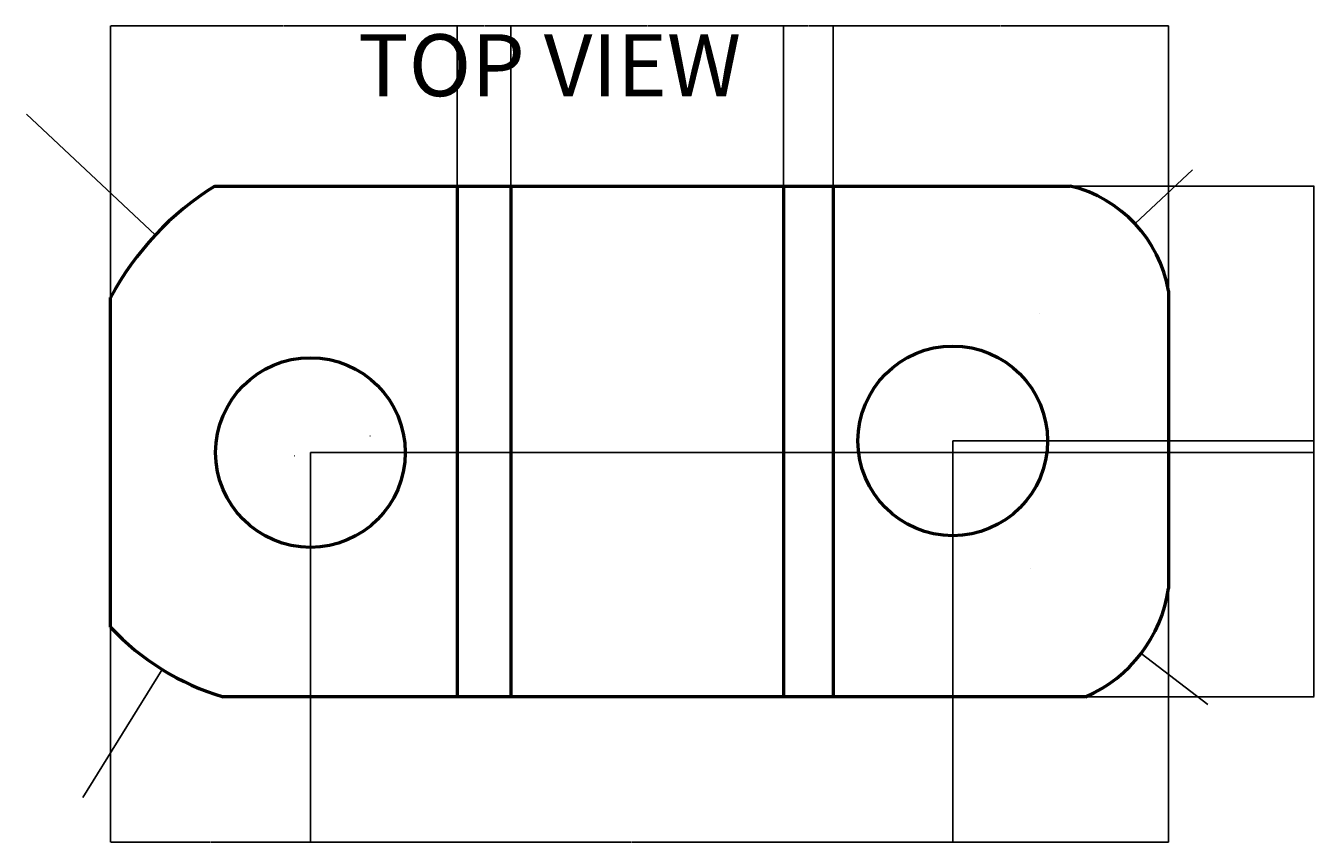
# Model space of a CAD drawing. Units: millimetres. Extents: x 647 to 5260, y 1116 to 2302.
# Tile 2 of 2: x 3387 to 5260, y 1116 to 2302. Entities that reach past the tile are written whole.
import ezdxf

# ---------------------------------------------------------------- set-up
doc = ezdxf.new("R2010")
doc.units = ezdxf.units.MM
for name, color, linetype, lineweight in [('M-DIMS', 2, 'Continuous', 18), ('M-OUTL', 7, 'Continuous', 50), ('M-TEXT', 3, 'Continuous', 25)]:
    doc.layers.add(name, color=color, linetype=linetype, lineweight=lineweight)
doc.styles.get("Standard").update_dxf_attribs({"font": 'arial.ttf'})
doc.dimstyles.get("Standard").update_dxf_attribs({"dimtxt": 0.18, "dimasz": 0.18, "dimexe": 0.18, "dimexo": 0.0625, "dimgap": 0.09, "dimtad": 0, "dimtih": 1, "dimtoh": 1, "dimdec": 4, "dimzin": 0, "dimdsep": 46, "dimtxsty": 'Standard', "dimcen": 0.09, "dimadec": 0, "dimazin": 0, "dimtfac": 1, "dimtdec": 4, "dimtofl": 0, "dimtmove": 0, "dimatfit": 3, "dimfxl": 1, "dimtolj": 1, "dimtzin": 0, "dimarcsym": 0})

# ---------------------------------------------------------------- blocks, each defined once
blk = doc.blocks.new('*D22')
at = {"layer": 'Defpoints', "color": 0, "transparency": 16777216}
for p in [(3800.8, 1681.9), (3510.3, 1428.3), (3800.8, 1116)]:
    blk.add_point(p, dxfattribs=at)
at = {"layer": 'M-DIMS', "color": 0, "lineweight": -2, "transparency": 16777216}
for p, q in [((3800.8, 1681.9), (3800.8, 1115.8)), ((3510.3, 1428.3), (3510.3, 1115.8)), ((3510.5, 1116), (3655.1, 1116)), ((3800.6, 1116), (3656, 1116))]:
    blk.add_line(p, q, dxfattribs=at)
at = {"layer": 'M-DIMS', "color": 0, "transparency": 16777216}
for points in [[(3510.5, 1116), (3510.5, 1115.9), (3510.3, 1116)], [(3800.6, 1116), (3800.6, 1115.9), (3800.8, 1116)]]:
    blk.add_solid(points, dxfattribs=at)
at = {"layer": 'M-DIMS', "color": 0, "transparency": 16777216, "insert": (3655.5, 1116), "char_height": 0.18, "attachment_point": 5}
blk.add_mtext('\\A1;290.45', dxfattribs=at)
blk = doc.blocks.new('*D23')
at = {"layer": 'Defpoints', "color": 0, "transparency": 16777216}
for p in [(4734.2, 1698.9), (3800.8, 1681.9), (4734.2, 1116)]:
    blk.add_point(p, dxfattribs=at)
at = {"layer": 'M-DIMS', "color": 0, "lineweight": -2, "transparency": 16777216}
for p, q in [((4734.2, 1698.8), (4734.2, 1115.8)), ((3800.8, 1681.9), (3800.8, 1115.8)), ((3800.9, 1116), (4267.1, 1116)), ((4734, 1116), (4267.9, 1116))]:
    blk.add_line(p, q, dxfattribs=at)
at = {"layer": 'M-DIMS', "color": 0, "transparency": 16777216}
for points in [[(3800.9, 1116), (3800.9, 1115.9), (3800.8, 1116)], [(4734, 1116), (4734, 1115.9), (4734.2, 1116)]]:
    blk.add_solid(points, dxfattribs=at)
at = {"layer": 'M-DIMS', "color": 0, "transparency": 16777216, "insert": (4267.5, 1116), "char_height": 0.18, "attachment_point": 5}
blk.add_mtext('\\A1;933.4', dxfattribs=at)
blk = doc.blocks.new('*D24')
at = {"layer": 'Defpoints', "color": 0, "transparency": 16777216}
for p in [(4734.2, 1698.9), (5047.9, 1484.3), (5047.9, 1116)]:
    blk.add_point(p, dxfattribs=at)
at = {"layer": 'M-DIMS', "color": 0, "lineweight": -2, "transparency": 16777216}
for p, q in [((4734.2, 1698.8), (4734.2, 1115.8)), ((5047.9, 1484.3), (5047.9, 1115.8)), ((4734.4, 1116), (4890.6, 1116)), ((5047.7, 1116), (4891.4, 1116))]:
    blk.add_line(p, q, dxfattribs=at)
at = {"layer": 'M-DIMS', "color": 0, "transparency": 16777216}
for points in [[(4734.4, 1116), (4734.4, 1115.9), (4734.2, 1116)], [(5047.7, 1116), (5047.7, 1115.9), (5047.9, 1116)]]:
    blk.add_solid(points, dxfattribs=at)
at = {"layer": 'M-DIMS', "color": 0, "transparency": 16777216, "insert": (4891, 1116), "char_height": 0.18, "attachment_point": 5}
blk.add_mtext('\\A1;313.7', dxfattribs=at)
blk = doc.blocks.new('*D25')
at = {"layer": 'Defpoints', "color": 0, "transparency": 16777216}
for p in [(4014.1, 2069.2), (5259.1, 2069.2), (4014.1, 1327.2)]:
    blk.add_point(p, dxfattribs=at)
at = {"layer": 'M-DIMS', "color": 0, "lineweight": -2, "transparency": 16777216}
for p, q in [((4014.1, 2069.2), (5259.3, 2069.2)), ((5259.1, 2069), (5259.1, 1698.4)), ((5259.1, 1327.4), (5259.1, 1698)), ((4014.1, 1327.2), (5259.3, 1327.2))]:
    blk.add_line(p, q, dxfattribs=at)
at = {"layer": 'M-DIMS', "color": 0, "transparency": 16777216}
for points in [[(5259.1, 2069), (5259.2, 2069), (5259.1, 2069.2)], [(5259.1, 1327.4), (5259.2, 1327.4), (5259.1, 1327.2)]]:
    blk.add_solid(points, dxfattribs=at)
at = {"layer": 'M-DIMS', "color": 0, "transparency": 16777216, "insert": (5259.1, 1698.2), "char_height": 0.18, "attachment_point": 5}
blk.add_mtext('\\A1;742', dxfattribs=at)
blk = doc.blocks.new('*D26')
at = {"layer": 'Defpoints', "color": 0, "transparency": 16777216}
for p in [(4014.1, 2069.2), (3800.8, 1681.9), (5259.1, 1681.9)]:
    blk.add_point(p, dxfattribs=at)
at = {"layer": 'M-DIMS', "color": 0, "lineweight": -2, "transparency": 16777216}
for p, q in [((4014.1, 2069.2), (5259.3, 2069.2)), ((5259.1, 2069), (5259.1, 1875.7)), ((5259.1, 1682.1), (5259.1, 1875.4)), ((3800.8, 1681.9), (5259.3, 1681.9))]:
    blk.add_line(p, q, dxfattribs=at)
at = {"layer": 'M-DIMS', "color": 0, "transparency": 16777216}
for points in [[(5259.1, 2069), (5259.2, 2069), (5259.1, 2069.2)], [(5259.1, 1682.1), (5259.2, 1682.1), (5259.1, 1681.9)]]:
    blk.add_solid(points, dxfattribs=at)
at = {"layer": 'M-DIMS', "color": 0, "transparency": 16777216, "insert": (5259.1, 1875.6), "char_height": 0.18, "attachment_point": 5}
blk.add_mtext('\\A1;387.3', dxfattribs=at)
blk = doc.blocks.new('*D27')
at = {"layer": 'Defpoints', "color": 0, "transparency": 16777216}
for p in [(4734.2, 1698.9), (5259.1, 1698.9), (4560.2, 1327.2)]:
    blk.add_point(p, dxfattribs=at)
at = {"layer": 'M-DIMS', "color": 0, "lineweight": -2, "transparency": 16777216}
for p, q in [((4734.2, 1698.9), (5259.3, 1698.9)), ((5259.1, 1698.7), (5259.1, 1513.2)), ((5259.1, 1327.4), (5259.1, 1512.9)), ((4560.3, 1327.2), (5259.3, 1327.2))]:
    blk.add_line(p, q, dxfattribs=at)
at = {"layer": 'M-DIMS', "color": 0, "transparency": 16777216}
for points in [[(5259.1, 1698.7), (5259.2, 1698.7), (5259.1, 1698.9)], [(5259.1, 1327.4), (5259.2, 1327.4), (5259.1, 1327.2)]]:
    blk.add_solid(points, dxfattribs=at)
at = {"layer": 'M-DIMS', "color": 0, "transparency": 16777216, "insert": (5259.1, 1513.1), "char_height": 0.18, "attachment_point": 5}
blk.add_mtext('\\A1;371.66', dxfattribs=at)
blk = doc.blocks.new('*D28')
at = {"layer": 'Defpoints', "color": 0, "transparency": 16777216}
for p in [(4014.1, 2301.8), (4014.1, 2069.2), (3510.3, 1907.2)]:
    blk.add_point(p, dxfattribs=at)
at = {"layer": 'M-DIMS', "color": 0, "lineweight": -2, "transparency": 16777216}
for p, q in [((3510.3, 1907.2), (3510.3, 2302)), ((3510.5, 2301.8), (3761.8, 2301.8)), ((4013.9, 2301.8), (3762.6, 2301.8)), ((4014.1, 2069.3), (4014.1, 2302))]:
    blk.add_line(p, q, dxfattribs=at)
at = {"layer": 'M-DIMS', "color": 0, "transparency": 16777216}
for points in [[(3510.5, 2301.9), (3510.5, 2301.8), (3510.3, 2301.8)], [(4013.9, 2301.9), (4013.9, 2301.8), (4014.1, 2301.8)]]:
    blk.add_solid(points, dxfattribs=at)
at = {"layer": 'M-DIMS', "color": 0, "transparency": 16777216, "insert": (3762.2, 2301.8), "char_height": 0.18, "attachment_point": 5}
blk.add_mtext('\\A1;503.8', dxfattribs=at)
blk = doc.blocks.new('*D29')
at = {"layer": 'Defpoints', "color": 0, "transparency": 16777216}
for p in [(4092.1, 2301.8), (4014.1, 2069.2), (4092.1, 2069.2)]:
    blk.add_point(p, dxfattribs=at)
at = {"layer": 'M-DIMS', "color": 0, "lineweight": -2, "transparency": 16777216}
for p, q in [((4014.1, 2069.3), (4014.1, 2302)), ((4014.2, 2301.8), (4052.7, 2301.8)), ((4091.9, 2301.8), (4053.5, 2301.8)), ((4092.1, 2069.3), (4092.1, 2302))]:
    blk.add_line(p, q, dxfattribs=at)
at = {"layer": 'M-DIMS', "color": 0, "transparency": 16777216}
for points in [[(4014.2, 2301.9), (4014.2, 2301.8), (4014.1, 2301.8)], [(4091.9, 2301.9), (4091.9, 2301.8), (4092.1, 2301.8)]]:
    blk.add_solid(points, dxfattribs=at)
at = {"layer": 'M-DIMS', "color": 0, "transparency": 16777216, "insert": (4053.1, 2301.8), "char_height": 0.18, "attachment_point": 5}
blk.add_mtext('\\A1;78.03', dxfattribs=at)
blk = doc.blocks.new('*D30')
at = {"layer": 'Defpoints', "color": 0, "transparency": 16777216}
for p in [(4488.2, 2301.8), (4092.1, 2069.2), (4488.2, 2069.2)]:
    blk.add_point(p, dxfattribs=at)
at = {"layer": 'M-DIMS', "color": 0, "lineweight": -2, "transparency": 16777216}
for p, q in [((4092.1, 2069.3), (4092.1, 2302)), ((4092.3, 2301.8), (4289.8, 2301.8)), ((4488, 2301.8), (4290.5, 2301.8)), ((4488.2, 2069.3), (4488.2, 2302))]:
    blk.add_line(p, q, dxfattribs=at)
at = {"layer": 'M-DIMS', "color": 0, "transparency": 16777216}
for points in [[(4092.3, 2301.9), (4092.3, 2301.8), (4092.1, 2301.8)], [(4488, 2301.9), (4488, 2301.8), (4488.2, 2301.8)]]:
    blk.add_solid(points, dxfattribs=at)
at = {"layer": 'M-DIMS', "color": 0, "transparency": 16777216, "insert": (4290.2, 2301.8), "char_height": 0.18, "attachment_point": 5}
blk.add_mtext('\\A1;396.1', dxfattribs=at)
blk = doc.blocks.new('*D31')
at = {"layer": 'Defpoints', "color": 0, "transparency": 16777216}
for p in [(4560.2, 2301.8), (4488.2, 2069.2), (4560.2, 2069.2)]:
    blk.add_point(p, dxfattribs=at)
at = {"layer": 'M-DIMS', "color": 0, "lineweight": -2, "transparency": 16777216}
for p, q in [((4488.2, 2069.3), (4488.2, 2302)), ((4488.4, 2301.8), (4523.8, 2301.8)), ((4560.1, 2301.8), (4524.6, 2301.8)), ((4560.2, 2069.3), (4560.2, 2302))]:
    blk.add_line(p, q, dxfattribs=at)
at = {"layer": 'M-DIMS', "color": 0, "transparency": 16777216}
for points in [[(4488.4, 2301.9), (4488.4, 2301.8), (4488.2, 2301.8)], [(4560.1, 2301.9), (4560.1, 2301.8), (4560.2, 2301.8)]]:
    blk.add_solid(points, dxfattribs=at)
at = {"layer": 'M-DIMS', "color": 0, "transparency": 16777216, "insert": (4524.2, 2301.8), "char_height": 0.18, "attachment_point": 5}
blk.add_mtext('\\A1;72.02', dxfattribs=at)
blk = doc.blocks.new('*D32')
at = {"layer": 'Defpoints', "color": 0, "transparency": 16777216}
for p in [(5047.9, 2301.8), (4560.2, 2069.2), (5047.9, 1917.1)]:
    blk.add_point(p, dxfattribs=at)
at = {"layer": 'M-DIMS', "color": 0, "lineweight": -2, "transparency": 16777216}
for p, q in [((4560.2, 2069.3), (4560.2, 2302)), ((4560.4, 2301.8), (4803.7, 2301.8)), ((5047.7, 2301.8), (4804.5, 2301.8)), ((5047.9, 1917.1), (5047.9, 2302))]:
    blk.add_line(p, q, dxfattribs=at)
at = {"layer": 'M-DIMS', "color": 0, "transparency": 16777216}
for points in [[(4560.4, 2301.9), (4560.4, 2301.8), (4560.2, 2301.8)], [(5047.7, 2301.9), (5047.7, 2301.8), (5047.9, 2301.8)]]:
    blk.add_solid(points, dxfattribs=at)
at = {"layer": 'M-DIMS', "color": 0, "transparency": 16777216, "insert": (4804.1, 2301.8), "char_height": 0.18, "attachment_point": 5}
blk.add_mtext('\\A1;487.6', dxfattribs=at)
blk = doc.blocks.new('*D36')
at = {"layer": 'Defpoints', "color": 0, "transparency": 16777216}
for p in [(3662.9, 1681.9), (3938.6, 1681.9)]:
    blk.add_point(p, dxfattribs=at)
at = {"layer": 'M-DIMS', "color": 0, "lineweight": -2, "transparency": 16777216}
for p, q in [((3800.7, 1681.9), (3800.8, 1681.9)), ((3800.8, 1681.8), (3800.8, 1682)), ((4021.2, 1681.9), (3938.7, 1681.9))]:
    blk.add_line(p, q, dxfattribs=at)
at = {"layer": 'M-DIMS', "color": 0, "transparency": 16777216}
blk.add_solid([(3938.7, 1681.9), (3938.7, 1681.9), (3938.6, 1681.9)], dxfattribs=at)
at = {"layer": 'M-DIMS', "color": 0, "transparency": 16777216, "insert": (4021.9, 1681.9), "char_height": 0.18, "attachment_point": 5}
blk.add_mtext('\\A1;2X ∅275.6', dxfattribs=at)
blk = doc.blocks.new('*D37')
at = {"layer": 'Defpoints', "color": 0, "transparency": 16777216}
for p in [(3575.5, 1998.2), (3887.6, 1705.9)]:
    blk.add_point(p, dxfattribs=at)
at = {"layer": 'M-DIMS', "color": 0, "lineweight": -2, "transparency": 16777216}
for p, q in [((3388, 2173.6), (3388.1, 2173.6)), ((3388.1, 2173.6), (3575.3, 1998.3)), ((3887.5, 1705.9), (3887.7, 1705.9)), ((3887.6, 1705.8), (3887.6, 1706))]:
    blk.add_line(p, q, dxfattribs=at)
at = {"layer": 'M-DIMS', "color": 0, "transparency": 16777216}
blk.add_solid([(3575.3, 1998.3), (3575.3, 1998.3), (3575.5, 1998.2)], dxfattribs=at)
at = {"layer": 'M-DIMS', "color": 0, "transparency": 16777216, "insert": (3387.5, 2173.6), "char_height": 0.18, "attachment_point": 5}
blk.add_mtext('\\A1;R427.6', dxfattribs=at)
blk = doc.blocks.new('*D38')
at = {"layer": 'Defpoints', "color": 0, "transparency": 16777216}
for p in [(3777.3, 1677.2), (3585.2, 1366.8)]:
    blk.add_point(p, dxfattribs=at)
at = {"layer": 'M-DIMS', "color": 0, "lineweight": -2, "transparency": 16777216}
for p, q in [((3777.2, 1677.2), (3777.4, 1677.2)), ((3777.3, 1677.1), (3777.3, 1677.3)), ((3470, 1180.6), (3585.2, 1366.7)), ((3469.9, 1180.6), (3470, 1180.6))]:
    blk.add_line(p, q, dxfattribs=at)
at = {"layer": 'M-DIMS', "color": 0, "transparency": 16777216}
blk.add_solid([(3585.1, 1366.7), (3585.2, 1366.7), (3585.2, 1366.8)], dxfattribs=at)
at = {"layer": 'M-DIMS', "color": 0, "transparency": 16777216, "insert": (3469.5, 1180.6), "char_height": 0.18, "attachment_point": 5}
blk.add_mtext('\\A1;R365', dxfattribs=at)
blk = doc.blocks.new('*D39')
at = {"layer": 'Defpoints', "color": 0, "transparency": 16777216}
for p in [(4846.7, 1514), (5008, 1390.1)]:
    blk.add_point(p, dxfattribs=at)
at = {"layer": 'M-DIMS', "color": 0, "lineweight": -2, "transparency": 16777216}
for p, q in [((4846.6, 1514), (4846.7, 1514)), ((4846.7, 1513.9), (4846.7, 1514.1)), ((5104.8, 1315.8), (5008.2, 1390)), ((5105, 1315.8), (5104.8, 1315.8))]:
    blk.add_line(p, q, dxfattribs=at)
at = {"layer": 'M-DIMS', "color": 0, "transparency": 16777216}
blk.add_solid([(5008.2, 1390), (5008.1, 1390), (5008, 1390.1)], dxfattribs=at)
at = {"layer": 'M-DIMS', "color": 0, "transparency": 16777216, "insert": (5105.5, 1315.8), "char_height": 0.18, "attachment_point": 5}
blk.add_mtext('\\A1;R203.4', dxfattribs=at)
blk = doc.blocks.new('*D40')
at = {"layer": 'Defpoints', "color": 0, "transparency": 16777216}
for p in [(4999.1, 2014.3), (4859.7, 1883.5)]:
    blk.add_point(p, dxfattribs=at)
at = {"layer": 'M-DIMS', "color": 0, "lineweight": -2, "transparency": 16777216}
for p, q in [((5082.7, 2092.8), (4999.2, 2014.5)), ((5082.8, 2092.8), (5082.7, 2092.8)), ((4859.6, 1883.5), (4859.8, 1883.5)), ((4859.7, 1883.4), (4859.7, 1883.6))]:
    blk.add_line(p, q, dxfattribs=at)
at = {"layer": 'M-DIMS', "color": 0, "transparency": 16777216}
blk.add_solid([(4999.2, 2014.5), (4999.2, 2014.4), (4999.1, 2014.3)], dxfattribs=at)
at = {"layer": 'M-DIMS', "color": 0, "transparency": 16777216, "insert": (5083.4, 2092.8), "char_height": 0.18, "attachment_point": 5}
blk.add_mtext('\\A1;R191.12', dxfattribs=at)

msp = doc.modelspace()

# ---------------------------------------------------------------- linework, layer by layer
at = {"layer": 'M-OUTL'}
for p, q in [((4014.066, 2069.1933), (4014.066, 1327.2273)), ((4014.066, 2069.1933), (4014.066, 1327.2273)), ((4092.092, 2069.1933), (4092.092, 1327.2273)), ((4488.2239, 2069.1933), (4488.2239, 1327.2273)), ((4560.2479, 2069.1933), (4560.2479, 1327.2273)), ((4560.2479, 2069.1933), (4560.2479, 1327.2273)), ((4560.2479, 2069.1933), (4560.2479, 1327.2273)), ((4560.2479, 2069.1933), (4560.2479, 1327.2273)), ((4560.2479, 2069.1933), (4560.2479, 1327.2273)), ((4560.2479, 2069.1933), (4560.2479, 1327.2273)), ((4560.2479, 2069.1933), (4560.2479, 1327.2273)), ((4560.2479, 2069.1933), (4560.2479, 1327.2273)), ((4560.2479, 2069.1933), (4560.2479, 1327.2273)), ((4560.2479, 2069.1933), (4560.2479, 1327.2273)), ((4560.2479, 2069.1933), (4560.2479, 1327.2273)), ((4560.2479, 2069.1933), (4560.2479, 1327.2273))]:
    msp.add_line(p, q, dxfattribs=at)
for points in [[(3661.9899, 2069.1933), (4905.062, 2069.1933)], [(5047.894, 1917.0715), (5047.894, 1484.3354)], [(3510.3005, 1428.3343), (3510.3005, 1907.1682)], [(4927.3089, 1327.2273), (3673.7422, 1327.2273)]]:
    msp.add_lwpolyline(points, dxfattribs=at)
for centre in [(4734.1808, 1698.8897), (3800.7513, 1681.9152)]:
    msp.add_circle(centre, 137.8065, dxfattribs=at)
for centre, radius, start, end in [((3887.6295, 1705.9284), 427.6384, 121.846209, 151.9277922), ((4859.74, 1883.5233), 191.1215, 10.1096915, 76.2823532), ((4846.6515, 1513.9646), 203.412, 293.3609366, 351.6244176), ((3777.2622, 1677.2266), 364.9875, 222.9938623, 253.5232552)]:
    msp.add_arc(centre, radius, start, end, dxfattribs=at)

# ---------------------------------------------------------------- texts
at = {"layer": 'M-TEXT', "insert": (3870.018, 2289.713), "char_height": 90, "attachment_point": 1}
msp.add_mtext('TOP VIEW', dxfattribs=at)

# ---------------------------------------------------------------- dimensions: what is measured, and where the dimension line sits
at = {"layer": 'M-DIMS'}
for base, p1, p2, override, picture, middle in [((4014.066, 2301.8231), (3510.3005, 1907.1682), (4014.066, 2069.1933), {"dimdec": 1, "dimlfac": 1, "dimrnd": 0, "dimzin": 0, "dimdsep": 46, "dimlunit": 2}, '*D28', (3762.1833, 2301.8231)), ((4092.092, 2301.8231), (4014.066, 2069.1933), (4092.092, 2069.1933), {"dimdec": 2, "dimlfac": 1, "dimrnd": 0, "dimzin": 0, "dimdsep": 46, "dimlunit": 2}, '*D29', (4053.079, 2301.8231)), ((4488.2239, 2301.8231), (4092.092, 2069.1933), (4488.2239, 2069.1933), {"dimdec": 1, "dimlfac": 1, "dimrnd": 0, "dimzin": 0, "dimdsep": 46, "dimlunit": 2}, '*D30', (4290.1579, 2301.8231)), ((4560.2479, 2301.8231), (4488.2239, 2069.1933), (4560.2479, 2069.1933), {"dimdec": 2, "dimlfac": 1, "dimrnd": 0, "dimzin": 0, "dimdsep": 46, "dimlunit": 2}, '*D31', (4524.2359, 2301.8231)), ((5047.894, 2301.8231), (4560.2479, 2069.1933), (5047.894, 1917.0715), {"dimdec": 1, "dimlfac": 1, "dimrnd": 0, "dimzin": 0, "dimdsep": 46, "dimlunit": 2}, '*D32', (4804.071, 2301.8231)), ((4734.1808, 1115.9773), (3800.7513, 1681.9152), (4734.1808, 1698.8897), {"dimdec": 1, "dimlfac": 1, "dimrnd": 0, "dimzin": 0, "dimdsep": 46, "dimlunit": 2}, '*D23', (4267.4661, 1115.9773)), ((5047.894, 1115.9773), (4734.1808, 1698.8897), (5047.894, 1484.3354), {"dimdec": 1, "dimlfac": 1, "dimrnd": 0, "dimzin": 0, "dimdsep": 46, "dimlunit": 2}, '*D24', (4891.0374, 1115.9773)), ((3800.7513, 1115.9773), (3510.3005, 1428.3343), (3800.7513, 1681.9152), {"dimdec": 2, "dimlfac": 1, "dimrnd": 0, "dimzin": 0, "dimdsep": 46, "dimlunit": 2}, '*D22', (3655.5259, 1115.9773))]:
    dim = msp.add_linear_dim(base=base, p1=p1, p2=p2, dimstyle='Standard', override=override, dxfattribs=at)
    dim.commit()
    dim.dimension.update_dxf_attribs({"geometry": picture, "text_midpoint": middle})
for center, mpoint, override, picture, middle in [((3887.6295, 1705.9284), (3575.45, 1998.193), {"dimdec": 1, "dimlfac": 1, "dimrnd": 0, "dimzin": 0, "dimdsep": 46, "dimlunit": 2}, '*D37', (3387.4826, 2173.5517)), ((4859.74, 1883.5233), (4999.071, 2014.345), {"dimdec": 2, "dimlfac": 1, "dimrnd": 0, "dimzin": 0, "dimdsep": 46, "dimlunit": 2}, '*D40', (5083.3984, 2092.838)), ((3777.2622, 1677.2266), (3585.247, 1366.83), {"dimdec": 0, "dimlfac": 1, "dimrnd": 0, "dimzin": 0, "dimdsep": 46, "dimlunit": 2}, '*D38', (3469.4822, 1180.592)), ((4846.6515, 1513.9646), (5008.0134, 1390.1147), {"dimdec": 1, "dimlfac": 1, "dimrnd": 0, "dimzin": 0, "dimdsep": 46, "dimlunit": 2}, '*D39', (5105.4899, 1315.8048))]:
    dim = msp.add_radius_dim(center=center, mpoint=mpoint, dimstyle='Standard', override=override, dxfattribs=at)
    dim.commit()
    dim.dimension.update_dxf_attribs({"geometry": picture, "text_midpoint": middle, "dimtype": 164})
for base, p1, p2, override, picture, middle in [((5259.144, 1681.9152), (4014.066, 2069.1933), (3800.7513, 1681.9152), {"dimdec": 1, "dimlfac": 1, "dimrnd": 0, "dimzin": 0, "dimdsep": 46, "dimlunit": 2}, '*D26', (5259.144, 1875.5542)), ((5259.144, 2069.1933), (4014.066, 1327.2273), (4014.066, 2069.1933), {"dimdec": 0, "dimlfac": 1, "dimrnd": 0, "dimzin": 0, "dimdsep": 46, "dimlunit": 2}, '*D25', (5259.144, 1698.2103)), ((5259.144, 1698.8897), (4560.2479, 1327.2273), (4734.1808, 1698.8897), {"dimdec": 2, "dimlfac": 1, "dimrnd": 0, "dimzin": 0, "dimdsep": 46, "dimlunit": 2}, '*D27', (5259.144, 1513.0585))]:
    dim = msp.add_linear_dim(base=base, p1=p1, p2=p2, angle=90, dimstyle='Standard', override=override, dxfattribs=at)
    dim.commit()
    dim.dimension.update_dxf_attribs({"geometry": picture, "text_midpoint": middle})
dim = msp.add_diameter_dim_2p(p1=(3662.9449, 1681.9154), p2=(3938.5578, 1681.915), text='2X <>', dimstyle='Standard', override={"dimdec": 1, "dimlfac": 1, "dimrnd": 0, "dimzin": 0, "dimdsep": 46, "dimlunit": 2}, dxfattribs=at)
dim.commit()
dim.dimension.update_dxf_attribs({"geometry": '*D36', "text_midpoint": (4021.2417, 1681.9149), "dimtype": 163})

doc.saveas('drawing.dxf')
